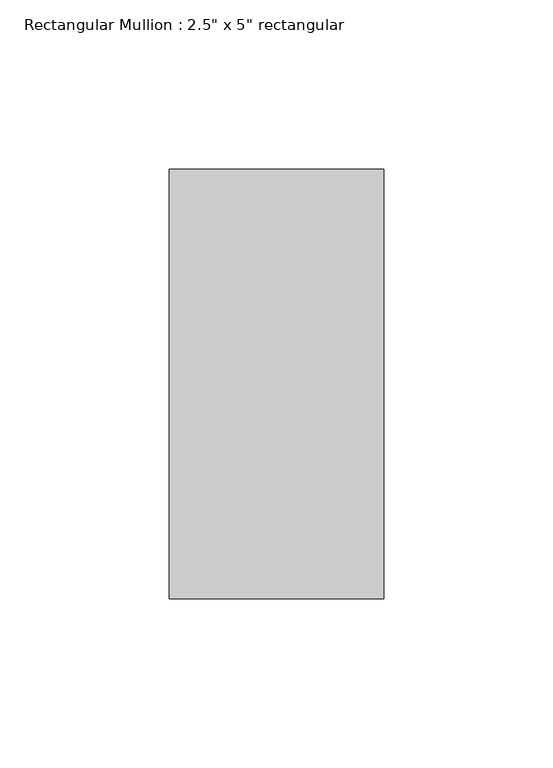
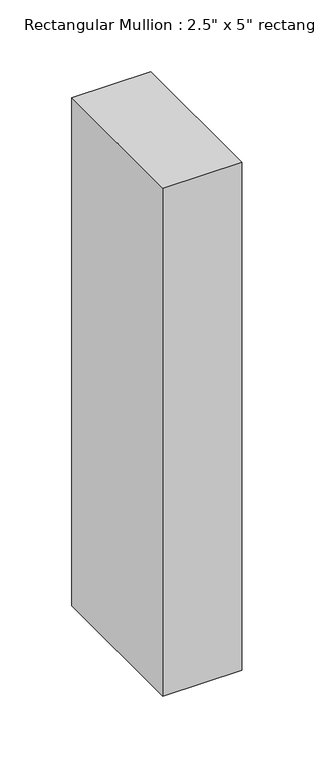
"""IFC4 building model written with IfcOpenShell, lengths in millimetres: member geometry."""

from ifc_helpers import new_model, si_unit, frame, origin, place, context, project, spatial, polyline, outline, extrude, source, transform, mapped, element, save


def member_69a911c1(model_context):
    return source(origin(), model_context, "Body", "SweptSolid", [
        extrude(outline(polyline([(0.0, 63.5), (0.0, -63.5), (-63.5, -63.5), (-63.5, 63.5), (0.0, 63.5)])), frame((0.0, 0.0, -431.8), z_axis=(0.0, 0.0, 1.0), x_axis=(1.0, 0.0, 0.0)), (0.0, 0.0, 1.0), 431.8),
    ])


if __name__ == "__main__":
    model = new_model("IFC4")
    model_context = context("Model", 3, world=origin())
    ifc_project = project(units=[si_unit("LENGTHUNIT", "METRE", prefix="MILLI")], contexts=[model_context])
    site = spatial("IfcSite", under=ifc_project)
    building = spatial("IfcBuilding", under=site)
    placement = place(None, origin())
    member_shape = member_69a911c1(model_context)
    element("IfcMember", 1, ObjectType="Rectangular Mullion : 2.5\" x 5\" rectangular", at=placement, inside=building, context=model_context, shape_type="MappedRepresentation", body=[
        mapped(member_shape, transform((0.0, 0.0, 0.0), x_axis=(1.0, 0.0, 0.0), y_axis=(0.0, 1.0, 0.0), z_axis=(0.0, 0.0, 1.0))),
    ])
    save(model, "model.ifc")

# Revit data of these elements
# Type "Rectangular Mullion : 2.5\" x 5\" rectangular"
#   built-in parameter 1007304 = 0.416667 (stored number, unit not read)
#   built-in parameter 1007301 = 0.104167 (stored number, unit not read)
#   built-in parameter 1007300 = 0.104167 (stored number, unit not read)
